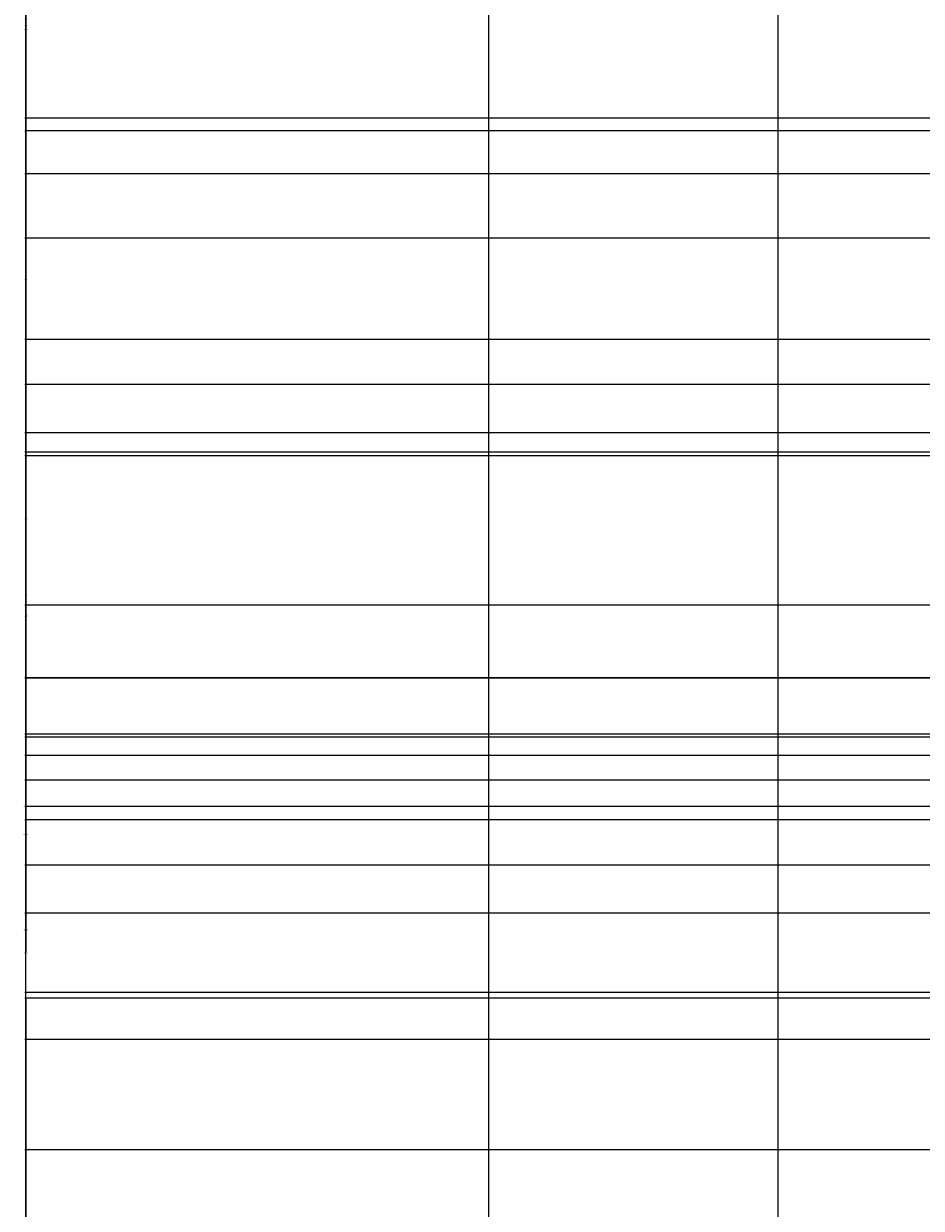
# Model space of a CAD drawing. Units: inches. Extents: x 818 to 1898, y 976 to 2364.
# Tile 5 of 96: x 818 to 986, y 1446 to 1668. Entities that reach past the tile are written whole.
import ezdxf

# ---------------------------------------------------------------- set-up
doc = ezdxf.new("R2010")
doc.units = ezdxf.units.IN
doc.header["$LTSCALE"] = 5
doc.header["$MEASUREMENT"] = 0
doc.layers.add('A-ANNO-DIMS', color=2, linetype='Continuous', lineweight=18)
doc.styles.get("Standard").update_dxf_attribs({"font": 'arial.ttf'})
doc.dimstyles.get("Standard").update_dxf_attribs({"dimtxt": 0.18, "dimasz": 0.18, "dimexe": 0.18, "dimexo": 0.0625, "dimgap": 0.09, "dimtad": 0, "dimtih": 1, "dimtoh": 1, "dimdec": 4, "dimzin": 0, "dimdsep": 46, "dimtxsty": 'Standard', "dimcen": 0.09, "dimadec": 0, "dimazin": 0, "dimtfac": 1, "dimtdec": 4, "dimtofl": 0, "dimtmove": 0, "dimatfit": 3, "dimfxl": 1, "dimtolj": 1, "dimtzin": 0, "dimarcsym": 0})

# ---------------------------------------------------------------- blocks, each defined once
blk = doc.blocks.new('*D59')
at = {"layer": 'A-ANNO-DIMS', "color": 0, "lineweight": -2, "ltscale": 5, "transparency": 16777216}
for p, q in [((1251.64, 2300.39), (818.03, 2300.39)), ((818.21, 2300.21), (818.21, 1669.95)), ((818.21, 1039.32), (818.21, 1669.59)), ((896.05, 1039.14), (818.03, 1039.14))]:
    blk.add_line(p, q, dxfattribs=at)
at = {"layer": 'A-ANNO-DIMS', "color": 0, "ltscale": 5, "transparency": 16777216}
for points in [[(818.18, 2300.21), (818.24, 2300.21), (818.21, 2300.39)], [(818.18, 1039.32), (818.24, 1039.32), (818.21, 1039.14)]]:
    blk.add_solid(points, dxfattribs=at)
at = {"layer": 'Defpoints', "color": 0, "ltscale": 5, "transparency": 16777216}
for p in [(818.21, 2300.39), (1251.71, 2300.39), (896.11, 1039.14)]:
    blk.add_point(p, dxfattribs=at)
at = {"layer": 'A-ANNO-DIMS', "color": 0, "ltscale": 5, "transparency": 16777216, "insert": (818.21, 1669.77), "char_height": 0.18, "attachment_point": 5}
blk.add_mtext('\\A1;1261.2', dxfattribs=at)
blk = doc.blocks.new('*D60')
at = {"layer": 'A-ANNO-DIMS', "color": 0, "lineweight": -2, "ltscale": 5, "transparency": 16777216}
for p, q in [((992.66, 2294.22), (818.03, 2294.22)), ((818.21, 2294.04), (818.21, 1748.77)), ((818.21, 1203.14), (818.21, 1748.41)), ((992.66, 1202.96), (818.03, 1202.96))]:
    blk.add_line(p, q, dxfattribs=at)
at = {"layer": 'A-ANNO-DIMS', "color": 0, "ltscale": 5, "transparency": 16777216}
for points in [[(818.18, 2294.04), (818.24, 2294.04), (818.21, 2294.22)], [(818.18, 1203.14), (818.24, 1203.14), (818.21, 1202.96)]]:
    blk.add_solid(points, dxfattribs=at)
at = {"layer": 'Defpoints', "color": 0, "ltscale": 5, "transparency": 16777216}
for p in [(818.21, 2294.22), (992.73, 2294.22), (992.73, 1202.96)]:
    blk.add_point(p, dxfattribs=at)
at = {"layer": 'A-ANNO-DIMS', "color": 0, "ltscale": 5, "transparency": 16777216, "insert": (818.21, 1748.59), "char_height": 0.18, "attachment_point": 5}
blk.add_mtext('\\A1;1091.3', dxfattribs=at)
blk = doc.blocks.new('*D63')
at = {"layer": 'A-ANNO-DIMS', "color": 0, "lineweight": -2, "ltscale": 5, "transparency": 16777216}
for p, q in [((1116.13, 1485.2), (818.03, 1485.2)), ((818.21, 1485.02), (818.21, 1360.77)), ((818.21, 1236.14), (818.21, 1360.4)), ((1116.13, 1235.96), (818.03, 1235.96))]:
    blk.add_line(p, q, dxfattribs=at)
at = {"layer": 'A-ANNO-DIMS', "color": 0, "ltscale": 5, "transparency": 16777216}
for points in [[(818.18, 1485.02), (818.24, 1485.02), (818.21, 1485.2)], [(818.18, 1236.14), (818.24, 1236.14), (818.21, 1235.96)]]:
    blk.add_solid(points, dxfattribs=at)
at = {"layer": 'Defpoints', "color": 0, "ltscale": 5, "transparency": 16777216}
for p in [(818.21, 1485.2), (1116.19, 1485.2), (1116.19, 1235.96)]:
    blk.add_point(p, dxfattribs=at)
at = {"layer": 'A-ANNO-DIMS', "color": 0, "ltscale": 5, "transparency": 16777216, "insert": (818.21, 1360.58), "char_height": 0.18, "attachment_point": 5}
blk.add_mtext('\\A1;249.24', dxfattribs=at)
blk = doc.blocks.new('*D84')
at = {"layer": 'A-ANNO-DIMS', "color": 0, "lineweight": -2, "ltscale": 5, "transparency": 16777216}
for p, q in [((1197.66, 1700.08), (818.03, 1700.08)), ((818.21, 1699.9), (818.21, 1600.76)), ((818.21, 1501.26), (818.21, 1600.4)), ((1197.66, 1501.08), (818.03, 1501.08))]:
    blk.add_line(p, q, dxfattribs=at)
at = {"layer": 'A-ANNO-DIMS', "color": 0, "ltscale": 5, "transparency": 16777216}
for points in [[(818.18, 1699.9), (818.24, 1699.9), (818.21, 1700.08)], [(818.18, 1501.26), (818.24, 1501.26), (818.21, 1501.08)]]:
    blk.add_solid(points, dxfattribs=at)
at = {"layer": 'Defpoints', "color": 0, "ltscale": 5, "transparency": 16777216}
for p in [(818.21, 1700.08), (1197.73, 1700.08), (1197.73, 1501.08)]:
    blk.add_point(p, dxfattribs=at)
at = {"layer": 'A-ANNO-DIMS', "color": 0, "ltscale": 5, "transparency": 16777216, "insert": (818.21, 1600.58), "char_height": 0.18, "attachment_point": 5}
blk.add_mtext('\\A1;199', dxfattribs=at)
blk = doc.blocks.new('*D90')
at = {"layer": 'A-ANNO-DIMS', "color": 0, "lineweight": -2, "ltscale": 5, "transparency": 16777216}
for p, q in [((904.95, 1071.12), (904.95, 2363.87)), ((905.13, 2363.69), (931.67, 2363.69)), ((958.99, 2363.69), (932.45, 2363.69)), ((959.17, 1071.12), (959.17, 2363.87))]:
    blk.add_line(p, q, dxfattribs=at)
at = {"layer": 'A-ANNO-DIMS', "color": 0, "ltscale": 5, "transparency": 16777216}
for points in [[(905.13, 2363.72), (905.13, 2363.66), (904.95, 2363.69)], [(958.99, 2363.72), (958.99, 2363.66), (959.17, 2363.69)]]:
    blk.add_solid(points, dxfattribs=at)
at = {"layer": 'Defpoints', "color": 0, "ltscale": 5, "transparency": 16777216}
for p in [(959.17, 2363.69), (904.95, 1071.06), (959.17, 1071.06)]:
    blk.add_point(p, dxfattribs=at)
at = {"layer": 'A-ANNO-DIMS', "color": 0, "ltscale": 5, "transparency": 16777216, "insert": (932.06, 2363.69), "char_height": 0.18, "attachment_point": 5}
blk.add_mtext('\\A1;54.22', dxfattribs=at)
blk = doc.blocks.new('*D91')
at = {"layer": 'A-ANNO-DIMS', "color": 0, "lineweight": -2, "ltscale": 5, "transparency": 16777216}
for p, q in [((959.17, 1071.12), (959.17, 2363.87)), ((959.35, 2363.69), (985.8, 2363.69)), ((1013.04, 2363.69), (986.59, 2363.69)), ((1013.22, 1071.12), (1013.22, 2363.87))]:
    blk.add_line(p, q, dxfattribs=at)
at = {"layer": 'A-ANNO-DIMS', "color": 0, "ltscale": 5, "transparency": 16777216}
for points in [[(959.35, 2363.72), (959.35, 2363.66), (959.17, 2363.69)], [(1013.04, 2363.72), (1013.04, 2363.66), (1013.22, 2363.69)]]:
    blk.add_solid(points, dxfattribs=at)
at = {"layer": 'Defpoints', "color": 0, "ltscale": 5, "transparency": 16777216}
for p in [(1013.22, 2363.69), (959.17, 1071.06), (1013.22, 1071.06)]:
    blk.add_point(p, dxfattribs=at)
at = {"layer": 'A-ANNO-DIMS', "color": 0, "ltscale": 5, "transparency": 16777216, "insert": (986.2, 2363.69), "char_height": 0.18, "attachment_point": 5}
blk.add_mtext('\\A1;54.04', dxfattribs=at)
blk = doc.blocks.new('*D116')
at = {"layer": 'A-ANNO-DIMS', "color": 0, "lineweight": -2, "ltscale": 5, "transparency": 16777216}
for p, q in [((1766.29, 1456.81), (818.03, 1456.81)), ((818.21, 1456.63), (818.21, 1417.41)), ((818.21, 1377.84), (818.21, 1417.05)), ((1766.29, 1377.66), (818.03, 1377.66))]:
    blk.add_line(p, q, dxfattribs=at)
at = {"layer": 'A-ANNO-DIMS', "color": 0, "ltscale": 5, "transparency": 16777216}
for points in [[(818.18, 1456.63), (818.24, 1456.63), (818.21, 1456.81)], [(818.18, 1377.84), (818.24, 1377.84), (818.21, 1377.66)]]:
    blk.add_solid(points, dxfattribs=at)
at = {"layer": 'Defpoints', "color": 0, "ltscale": 5, "transparency": 16777216}
for p in [(818.21, 1456.81), (1766.35, 1456.81), (1766.35, 1377.66)]:
    blk.add_point(p, dxfattribs=at)
at = {"layer": 'A-ANNO-DIMS', "color": 0, "ltscale": 5, "transparency": 16777216, "insert": (818.21, 1417.23), "char_height": 0.18, "attachment_point": 5}
blk.add_mtext('\\A1;79.15', dxfattribs=at)
blk = doc.blocks.new('*D117')
at = {"layer": 'A-ANNO-DIMS', "color": 0, "lineweight": -2, "ltscale": 5, "transparency": 16777216}
for p, q in [((1766.29, 1545.18), (818.03, 1545.18)), ((818.21, 1545), (818.21, 1501.18)), ((818.21, 1456.99), (818.21, 1500.81)), ((1766.29, 1456.81), (818.03, 1456.81))]:
    blk.add_line(p, q, dxfattribs=at)
at = {"layer": 'A-ANNO-DIMS', "color": 0, "ltscale": 5, "transparency": 16777216}
for points in [[(818.18, 1545), (818.24, 1545), (818.21, 1545.18)], [(818.18, 1456.99), (818.24, 1456.99), (818.21, 1456.81)]]:
    blk.add_solid(points, dxfattribs=at)
at = {"layer": 'Defpoints', "color": 0, "ltscale": 5, "transparency": 16777216}
for p in [(818.21, 1545.18), (1766.35, 1545.18), (1766.35, 1456.81)]:
    blk.add_point(p, dxfattribs=at)
at = {"layer": 'A-ANNO-DIMS', "color": 0, "ltscale": 5, "transparency": 16777216, "insert": (818.21, 1501), "char_height": 0.18, "attachment_point": 5}
blk.add_mtext('\\A1;88.37', dxfattribs=at)
blk = doc.blocks.new('*D118')
at = {"layer": 'A-ANNO-DIMS', "color": 0, "lineweight": -2, "ltscale": 5, "transparency": 16777216}
for p, q in [((1766.29, 1627.51), (818.03, 1627.51)), ((818.21, 1627.33), (818.21, 1586.53)), ((818.21, 1545.36), (818.21, 1586.16)), ((1766.29, 1545.18), (818.03, 1545.18))]:
    blk.add_line(p, q, dxfattribs=at)
at = {"layer": 'A-ANNO-DIMS', "color": 0, "ltscale": 5, "transparency": 16777216}
for points in [[(818.18, 1627.33), (818.24, 1627.33), (818.21, 1627.51)], [(818.18, 1545.36), (818.24, 1545.36), (818.21, 1545.18)]]:
    blk.add_solid(points, dxfattribs=at)
at = {"layer": 'Defpoints', "color": 0, "ltscale": 5, "transparency": 16777216}
for p in [(818.21, 1627.51), (1766.35, 1627.51), (1766.35, 1545.18)]:
    blk.add_point(p, dxfattribs=at)
at = {"layer": 'A-ANNO-DIMS', "color": 0, "ltscale": 5, "transparency": 16777216, "insert": (818.21, 1586.34), "char_height": 0.18, "attachment_point": 5}
blk.add_mtext('\\A1;82.32', dxfattribs=at)
blk = doc.blocks.new('*D119')
at = {"layer": 'A-ANNO-DIMS', "color": 0, "lineweight": -2, "ltscale": 5, "transparency": 16777216}
for p, q in [((1766.29, 1716.99), (818.03, 1716.99)), ((818.21, 1716.81), (818.21, 1672.43)), ((818.21, 1627.69), (818.21, 1672.06)), ((1766.29, 1627.51), (818.03, 1627.51))]:
    blk.add_line(p, q, dxfattribs=at)
at = {"layer": 'A-ANNO-DIMS', "color": 0, "ltscale": 5, "transparency": 16777216}
for points in [[(818.18, 1716.81), (818.24, 1716.81), (818.21, 1716.99)], [(818.18, 1627.69), (818.24, 1627.69), (818.21, 1627.51)]]:
    blk.add_solid(points, dxfattribs=at)
at = {"layer": 'Defpoints', "color": 0, "ltscale": 5, "transparency": 16777216}
for p in [(818.21, 1716.99), (1766.35, 1716.99), (1766.35, 1627.51)]:
    blk.add_point(p, dxfattribs=at)
at = {"layer": 'A-ANNO-DIMS', "color": 0, "ltscale": 5, "transparency": 16777216, "insert": (818.21, 1672.25), "char_height": 0.18, "attachment_point": 5}
blk.add_mtext('\\A1;89.48', dxfattribs=at)
blk = doc.blocks.new('*D129')
at = {"layer": 'A-ANNO-DIMS', "color": 0, "lineweight": -2, "ltscale": 5, "transparency": 16777216}
for p, q in [((1044.78, 1608.51), (818.03, 1608.51)), ((818.21, 1608.33), (818.21, 1521.27)), ((818.21, 1433.85), (818.21, 1520.91)), ((1044.78, 1433.67), (818.03, 1433.67))]:
    blk.add_line(p, q, dxfattribs=at)
at = {"layer": 'A-ANNO-DIMS', "color": 0, "ltscale": 5, "transparency": 16777216}
for points in [[(818.18, 1608.33), (818.24, 1608.33), (818.21, 1608.51)], [(818.18, 1433.85), (818.24, 1433.85), (818.21, 1433.67)]]:
    blk.add_solid(points, dxfattribs=at)
at = {"layer": 'Defpoints', "color": 0, "ltscale": 5, "transparency": 16777216}
for p in [(818.21, 1608.51), (1044.85, 1608.51), (1044.85, 1433.67)]:
    blk.add_point(p, dxfattribs=at)
at = {"layer": 'A-ANNO-DIMS', "color": 0, "ltscale": 5, "transparency": 16777216, "insert": (818.21, 1521.09), "char_height": 0.18, "attachment_point": 5}
blk.add_mtext('\\A1;174.84', dxfattribs=at)
blk = doc.blocks.new('*D130')
at = {"layer": 'A-ANNO-DIMS', "color": 0, "lineweight": -2, "ltscale": 5, "transparency": 16777216}
for p, q in [((1044.78, 1724.63), (818.03, 1724.63)), ((818.21, 1724.45), (818.21, 1666.75)), ((818.21, 1608.69), (818.21, 1666.39)), ((1044.78, 1608.51), (818.03, 1608.51))]:
    blk.add_line(p, q, dxfattribs=at)
at = {"layer": 'A-ANNO-DIMS', "color": 0, "ltscale": 5, "transparency": 16777216}
for points in [[(818.18, 1724.45), (818.24, 1724.45), (818.21, 1724.63)], [(818.18, 1608.69), (818.24, 1608.69), (818.21, 1608.51)]]:
    blk.add_solid(points, dxfattribs=at)
at = {"layer": 'Defpoints', "color": 0, "ltscale": 5, "transparency": 16777216}
for p in [(818.21, 1724.63), (1044.85, 1724.63), (1044.85, 1608.51)]:
    blk.add_point(p, dxfattribs=at)
at = {"layer": 'A-ANNO-DIMS', "color": 0, "ltscale": 5, "transparency": 16777216, "insert": (818.21, 1666.57), "char_height": 0.18, "attachment_point": 5}
blk.add_mtext('\\A1;116.12', dxfattribs=at)
blk = doc.blocks.new('*D156')
at = {"layer": 'A-ANNO-DIMS', "color": 0, "lineweight": -2, "ltscale": 5, "transparency": 16777216}
for p, q in [((1177.66, 1586.76), (818.03, 1586.76)), ((818.21, 1586.58), (818.21, 1560.86)), ((818.21, 1534.78), (818.21, 1560.5)), ((1177.66, 1534.6), (818.03, 1534.6))]:
    blk.add_line(p, q, dxfattribs=at)
at = {"layer": 'A-ANNO-DIMS', "color": 0, "ltscale": 5, "transparency": 16777216}
for points in [[(818.18, 1586.58), (818.24, 1586.58), (818.21, 1586.76)], [(818.18, 1534.78), (818.24, 1534.78), (818.21, 1534.6)]]:
    blk.add_solid(points, dxfattribs=at)
at = {"layer": 'Defpoints', "color": 0, "ltscale": 5, "transparency": 16777216}
for p in [(818.21, 1586.76), (1177.73, 1586.76), (1177.73, 1534.6)]:
    blk.add_point(p, dxfattribs=at)
at = {"layer": 'A-ANNO-DIMS', "color": 0, "ltscale": 5, "transparency": 16777216, "insert": (818.21, 1560.68), "char_height": 0.18, "attachment_point": 5}
blk.add_mtext('\\A1;52.16', dxfattribs=at)
blk = doc.blocks.new('*D157')
at = {"layer": 'A-ANNO-DIMS', "color": 0, "lineweight": -2, "ltscale": 5, "transparency": 16777216}
for p, q in [((1197.66, 1530.6), (818.03, 1530.6)), ((818.21, 1530.42), (818.21, 1516.02)), ((818.21, 1501.26), (818.21, 1515.66)), ((1197.66, 1501.08), (818.03, 1501.08))]:
    blk.add_line(p, q, dxfattribs=at)
at = {"layer": 'A-ANNO-DIMS', "color": 0, "ltscale": 5, "transparency": 16777216}
for points in [[(818.18, 1530.42), (818.24, 1530.42), (818.21, 1530.6)], [(818.18, 1501.26), (818.24, 1501.26), (818.21, 1501.08)]]:
    blk.add_solid(points, dxfattribs=at)
at = {"layer": 'Defpoints', "color": 0, "ltscale": 5, "transparency": 16777216}
for p in [(818.21, 1530.6), (1197.73, 1530.6), (1197.73, 1501.08)]:
    blk.add_point(p, dxfattribs=at)
at = {"layer": 'A-ANNO-DIMS', "color": 0, "ltscale": 5, "transparency": 16777216, "insert": (818.21, 1515.84), "char_height": 0.18, "attachment_point": 5}
blk.add_mtext('\\A1;29.524', dxfattribs=at)
blk = doc.blocks.new('*D168')
at = {"layer": 'A-ANNO-DIMS', "color": 0, "lineweight": -2, "ltscale": 5, "transparency": 16777216}
for p, q in [((1430.66, 1501.08), (818.03, 1501.08)), ((818.21, 1500.9), (818.21, 1493.84)), ((818.21, 1486.42), (818.21, 1493.48)), ((1430.66, 1486.24), (818.03, 1486.24))]:
    blk.add_line(p, q, dxfattribs=at)
at = {"layer": 'A-ANNO-DIMS', "color": 0, "ltscale": 5, "transparency": 16777216}
for points in [[(818.18, 1500.9), (818.24, 1500.9), (818.21, 1501.08)], [(818.18, 1486.42), (818.24, 1486.42), (818.21, 1486.24)]]:
    blk.add_solid(points, dxfattribs=at)
at = {"layer": 'Defpoints', "color": 0, "ltscale": 5, "transparency": 16777216}
for p in [(818.21, 1501.08), (1430.73, 1501.08), (1430.73, 1486.24)]:
    blk.add_point(p, dxfattribs=at)
at = {"layer": 'A-ANNO-DIMS', "color": 0, "ltscale": 5, "transparency": 16777216, "insert": (818.21, 1493.66), "char_height": 0.18, "attachment_point": 5}
blk.add_mtext('\\A1;14.84', dxfattribs=at)
blk = doc.blocks.new('*D176')
at = {"layer": 'A-ANNO-DIMS', "color": 0, "lineweight": -2, "ltscale": 5, "transparency": 16777216}
for p, q in [((1559.66, 1687.08), (818.03, 1687.08)), ((818.21, 1686.9), (818.21, 1667.51)), ((818.21, 1647.76), (818.21, 1667.15)), ((1559.66, 1647.58), (818.03, 1647.58))]:
    blk.add_line(p, q, dxfattribs=at)
at = {"layer": 'A-ANNO-DIMS', "color": 0, "ltscale": 5, "transparency": 16777216}
for points in [[(818.18, 1686.9), (818.24, 1686.9), (818.21, 1687.08)], [(818.18, 1647.76), (818.24, 1647.76), (818.21, 1647.58)]]:
    blk.add_solid(points, dxfattribs=at)
at = {"layer": 'Defpoints', "color": 0, "ltscale": 5, "transparency": 16777216}
for p in [(1559.73, 1687.08), (818.21, 1647.58), (1559.73, 1647.58)]:
    blk.add_point(p, dxfattribs=at)
at = {"layer": 'A-ANNO-DIMS', "color": 0, "ltscale": 5, "transparency": 16777216, "insert": (818.21, 1667.33), "char_height": 0.18, "attachment_point": 5}
blk.add_mtext('\\A1;39.5', dxfattribs=at)
blk = doc.blocks.new('*D181')
at = {"layer": 'A-ANNO-DIMS', "color": 0, "lineweight": -2, "ltscale": 5, "transparency": 16777216}
for p, q in [((1599.66, 1639.58), (818.03, 1639.58)), ((818.21, 1639.4), (818.21, 1620.01)), ((818.21, 1600.26), (818.21, 1619.65)), ((1619.66, 1600.08), (818.03, 1600.08))]:
    blk.add_line(p, q, dxfattribs=at)
at = {"layer": 'A-ANNO-DIMS', "color": 0, "ltscale": 5, "transparency": 16777216}
for points in [[(818.18, 1639.4), (818.24, 1639.4), (818.21, 1639.58)], [(818.18, 1600.26), (818.24, 1600.26), (818.21, 1600.08)]]:
    blk.add_solid(points, dxfattribs=at)
at = {"layer": 'Defpoints', "color": 0, "ltscale": 5, "transparency": 16777216}
for p in [(1599.73, 1639.58), (818.21, 1600.08), (1619.73, 1600.08)]:
    blk.add_point(p, dxfattribs=at)
at = {"layer": 'A-ANNO-DIMS', "color": 0, "ltscale": 5, "transparency": 16777216, "insert": (818.21, 1619.83), "char_height": 0.18, "attachment_point": 5}
blk.add_mtext('\\A1;39.5', dxfattribs=at)
blk = doc.blocks.new('*D187')
at = {"layer": 'A-ANNO-DIMS', "color": 0, "lineweight": -2, "ltscale": 5, "transparency": 16777216}
for p, q in [((1705.66, 1545.08), (818.03, 1545.08)), ((818.21, 1544.9), (818.21, 1533.26)), ((818.21, 1521.26), (818.21, 1532.9)), ((1705.66, 1521.08), (818.03, 1521.08))]:
    blk.add_line(p, q, dxfattribs=at)
at = {"layer": 'A-ANNO-DIMS', "color": 0, "ltscale": 5, "transparency": 16777216}
for points in [[(818.18, 1544.9), (818.24, 1544.9), (818.21, 1545.08)], [(818.18, 1521.26), (818.24, 1521.26), (818.21, 1521.08)]]:
    blk.add_solid(points, dxfattribs=at)
at = {"layer": 'Defpoints', "color": 0, "ltscale": 5, "transparency": 16777216}
for p in [(818.21, 1545.08), (1705.73, 1545.08), (1705.73, 1521.08)]:
    blk.add_point(p, dxfattribs=at)
at = {"layer": 'A-ANNO-DIMS', "color": 0, "ltscale": 5, "transparency": 16777216, "insert": (818.21, 1533.08), "char_height": 0.18, "attachment_point": 5}
blk.add_mtext('\\A1;24', dxfattribs=at)
blk = doc.blocks.new('*D194')
at = {"layer": 'A-ANNO-DIMS', "color": 0, "lineweight": -2, "ltscale": 5, "transparency": 16777216}
for p, q in [((1616.66, 1591.08), (818.03, 1591.08)), ((818.21, 1590.9), (818.21, 1575.1)), ((818.21, 1558.93), (818.21, 1574.73)), ((1616.66, 1558.75), (818.03, 1558.75))]:
    blk.add_line(p, q, dxfattribs=at)
at = {"layer": 'A-ANNO-DIMS', "color": 0, "ltscale": 5, "transparency": 16777216}
for points in [[(818.18, 1590.9), (818.24, 1590.9), (818.21, 1591.08)], [(818.18, 1558.93), (818.24, 1558.93), (818.21, 1558.75)]]:
    blk.add_solid(points, dxfattribs=at)
at = {"layer": 'Defpoints', "color": 0, "ltscale": 5, "transparency": 16777216}
for p in [(818.21, 1591.08), (1616.73, 1591.08), (1616.73, 1558.75)]:
    blk.add_point(p, dxfattribs=at)
at = {"layer": 'A-ANNO-DIMS', "color": 0, "ltscale": 5, "transparency": 16777216, "insert": (818.21, 1574.92), "char_height": 0.18, "attachment_point": 5}
blk.add_mtext('\\A1;32.326', dxfattribs=at)
blk = doc.blocks.new('*D201')
at = {"layer": 'A-ANNO-DIMS', "color": 0, "lineweight": -2, "ltscale": 5, "transparency": 16777216}
for p, q in [((1678.27, 1518.56), (818.03, 1518.56)), ((818.21, 1518.38), (818.21, 1498.18)), ((818.21, 1477.61), (818.21, 1497.81)), ((1678.27, 1477.43), (818.03, 1477.43))]:
    blk.add_line(p, q, dxfattribs=at)
at = {"layer": 'A-ANNO-DIMS', "color": 0, "ltscale": 5, "transparency": 16777216}
for points in [[(818.18, 1518.38), (818.24, 1518.38), (818.21, 1518.56)], [(818.18, 1477.61), (818.24, 1477.61), (818.21, 1477.43)]]:
    blk.add_solid(points, dxfattribs=at)
at = {"layer": 'Defpoints', "color": 0, "ltscale": 5, "transparency": 16777216}
for p in [(818.21, 1518.56), (1678.33, 1518.56), (1678.33, 1477.43)]:
    blk.add_point(p, dxfattribs=at)
at = {"layer": 'A-ANNO-DIMS', "color": 0, "ltscale": 5, "transparency": 16777216, "insert": (818.21, 1497.99), "char_height": 0.18, "attachment_point": 5}
blk.add_mtext('\\A1;41.135', dxfattribs=at)
blk = doc.blocks.new('*D270')
at = {"layer": 'A-ANNO-DIMS', "color": 0, "lineweight": -2, "ltscale": 5, "transparency": 16777216}
for p, q in [((1246.88, 1534.08), (818.03, 1534.08)), ((818.21, 1533.9), (818.21, 1522.26)), ((818.21, 1510.26), (818.21, 1521.9)), ((1246.88, 1510.08), (818.03, 1510.08))]:
    blk.add_line(p, q, dxfattribs=at)
at = {"layer": 'A-ANNO-DIMS', "color": 0, "ltscale": 5, "transparency": 16777216}
for points in [[(818.18, 1533.9), (818.24, 1533.9), (818.21, 1534.08)], [(818.18, 1510.26), (818.24, 1510.26), (818.21, 1510.08)]]:
    blk.add_solid(points, dxfattribs=at)
at = {"layer": 'Defpoints', "color": 0, "ltscale": 5, "transparency": 16777216}
for p in [(818.21, 1534.08), (1246.94, 1534.08), (1246.94, 1510.08)]:
    blk.add_point(p, dxfattribs=at)
at = {"layer": 'A-ANNO-DIMS', "color": 0, "ltscale": 5, "transparency": 16777216, "insert": (818.21, 1522.08), "char_height": 0.18, "attachment_point": 5}
blk.add_mtext('\\A1;24', dxfattribs=at)
blk = doc.blocks.new('*D272')
at = {"layer": 'A-ANNO-DIMS', "color": 0, "lineweight": -2, "ltscale": 5, "transparency": 16777216}
for p, q in [((1406.66, 1587.42), (818.03, 1587.42)), ((818.21, 1587.24), (818.21, 1556.89)), ((818.21, 1526.18), (818.21, 1556.52)), ((1406.66, 1526), (818.03, 1526))]:
    blk.add_line(p, q, dxfattribs=at)
at = {"layer": 'A-ANNO-DIMS', "color": 0, "ltscale": 5, "transparency": 16777216}
for points in [[(818.18, 1587.24), (818.24, 1587.24), (818.21, 1587.42)], [(818.18, 1526.18), (818.24, 1526.18), (818.21, 1526)]]:
    blk.add_solid(points, dxfattribs=at)
at = {"layer": 'Defpoints', "color": 0, "ltscale": 5, "transparency": 16777216}
for p in [(818.21, 1587.42), (1406.73, 1587.42), (1406.73, 1526)]:
    blk.add_point(p, dxfattribs=at)
at = {"layer": 'A-ANNO-DIMS', "color": 0, "ltscale": 5, "transparency": 16777216, "insert": (818.21, 1556.71), "char_height": 0.18, "attachment_point": 5}
blk.add_mtext('\\A1;61.42', dxfattribs=at)
blk = doc.blocks.new('*D277')
at = {"layer": 'A-ANNO-DIMS', "color": 0, "lineweight": -2, "ltscale": 5, "transparency": 16777216}
for p, q in [((1251.87, 1687.08), (818.03, 1687.08)), ((818.21, 1686.9), (818.21, 1668.7)), ((818.21, 1650.13), (818.21, 1668.33)), ((1256.59, 1649.95), (818.03, 1649.95))]:
    blk.add_line(p, q, dxfattribs=at)
at = {"layer": 'A-ANNO-DIMS', "color": 0, "ltscale": 5, "transparency": 16777216}
for points in [[(818.18, 1686.9), (818.24, 1686.9), (818.21, 1687.08)], [(818.18, 1650.13), (818.24, 1650.13), (818.21, 1649.95)]]:
    blk.add_solid(points, dxfattribs=at)
at = {"layer": 'Defpoints', "color": 0, "ltscale": 5, "transparency": 16777216}
for p in [(818.21, 1687.08), (1251.93, 1687.08), (1256.65, 1649.95)]:
    blk.add_point(p, dxfattribs=at)
at = {"layer": 'A-ANNO-DIMS', "color": 0, "ltscale": 5, "transparency": 16777216, "insert": (818.21, 1668.52), "char_height": 0.18, "attachment_point": 5}
blk.add_mtext('\\A1;37.13', dxfattribs=at)

msp = doc.modelspace()

# ---------------------------------------------------------------- dimensions: what is measured, and where the dimension line sits
at = {"layer": 'A-ANNO-DIMS', "ltscale": 5}
for base, p1, p2, picture, middle in [((959.1737, 2363.6929), (904.9504, 1071.0552), (959.1737, 1071.0552), '*D90', (932.062, 2363.6929)), ((1013.2176, 2363.6929), (959.1737, 1071.0552), (1013.2176, 1071.0552), '*D91', (986.1956, 2363.6929))]:
    dim = msp.add_linear_dim(base=base, p1=p1, p2=p2, dimstyle='Standard', override={"dimdec": 2, "dimlfac": 1, "dimrnd": 0, "dimzin": 0, "dimdsep": 46, "dimlunit": 2}, dxfattribs=at)
    dim.commit()
    dim.dimension.update_dxf_attribs({"geometry": picture, "text_midpoint": middle})
for base, p1, p2, override, picture, middle in [((818.2059, 2300.3929), (896.1138, 1039.1433), (1251.7057, 2300.3929), {"dimdec": 1, "dimlfac": 1, "dimrnd": 0, "dimzin": 0, "dimdsep": 46, "dimlunit": 2}, '*D59', (818.2059, 1669.7681)), ((818.2059, 2294.2171), (992.7251, 1202.9642), (992.7251, 2294.2171), {"dimdec": 1, "dimlfac": 1, "dimrnd": 0, "dimzin": 0, "dimdsep": 46, "dimlunit": 2}, '*D60', (818.2059, 1748.5907)), ((818.2059, 1724.63), (1044.8463, 1608.5116), (1044.8463, 1724.63), {"dimdec": 2, "dimlfac": 1, "dimrnd": 0, "dimzin": 0, "dimdsep": 46, "dimlunit": 2}, '*D130', (818.2059, 1666.5708)), ((818.2059, 1716.9866), (1766.3524, 1627.5052), (1766.3524, 1716.9866), {"dimdec": 2, "dimlfac": 1, "dimrnd": 0, "dimzin": 0, "dimdsep": 46, "dimlunit": 2}, '*D119', (818.2059, 1672.2459)), ((818.2059, 1700.0782), (1197.7251, 1501.0782), (1197.7251, 1700.0782), {"dimdec": 0, "dimlfac": 1, "dimrnd": 0, "dimzin": 0, "dimdsep": 46, "dimlunit": 2}, '*D84', (818.2059, 1600.5782)), ((818.2059, 1687.0782), (1256.6519, 1649.9518), (1251.9333, 1687.0782), {"dimdec": 2, "dimlfac": 1, "dimrnd": 0, "dimzin": 0, "dimdsep": 46, "dimlunit": 2}, '*D277', (818.2059, 1668.515)), ((818.2059, 1647.5782), (1559.7251, 1687.0782), (1559.7251, 1647.5782), {"dimdec": 1, "dimlfac": 1, "dimrnd": 0, "dimzin": 0, "dimdsep": 46, "dimlunit": 2}, '*D176', (818.2059, 1667.3282)), ((818.2059, 1600.0782), (1599.7251, 1639.5782), (1619.7251, 1600.0782), {"dimdec": 1, "dimlfac": 1, "dimrnd": 0, "dimzin": 0, "dimdsep": 46, "dimlunit": 2}, '*D181', (818.2059, 1619.8282)), ((818.2059, 1627.5052), (1766.3524, 1545.1827), (1766.3524, 1627.5052), {"dimdec": 2, "dimlfac": 1, "dimrnd": 0, "dimzin": 0, "dimdsep": 46, "dimlunit": 2}, '*D118', (818.2059, 1586.3439)), ((818.2059, 1608.5116), (1044.8463, 1433.6672), (1044.8463, 1608.5116), {"dimdec": 2, "dimlfac": 1, "dimrnd": 0, "dimzin": 0, "dimdsep": 46, "dimlunit": 2}, '*D129', (818.2059, 1521.0894)), ((818.2059, 1591.0782), (1616.7251, 1558.7521), (1616.7251, 1591.0782), {"dimdec": 3, "dimlfac": 1, "dimrnd": 0, "dimzin": 0, "dimdsep": 46, "dimlunit": 2}, '*D194', (818.2059, 1574.9152)), ((818.2059, 1587.4164), (1406.7251, 1525.9965), (1406.7251, 1587.4164), {"dimdec": 2, "dimlfac": 1, "dimrnd": 0, "dimzin": 0, "dimdsep": 46, "dimlunit": 2}, '*D272', (818.2059, 1556.7064)), ((818.2059, 1586.7585), (1177.7251, 1534.6024), (1177.7251, 1586.7585), {"dimdec": 2, "dimlfac": 1, "dimrnd": 0, "dimzin": 0, "dimdsep": 46, "dimlunit": 2}, '*D156', (818.2059, 1560.6805)), ((818.2059, 1545.1827), (1766.3524, 1456.8088), (1766.3524, 1545.1827), {"dimdec": 2, "dimlfac": 1, "dimrnd": 0, "dimzin": 0, "dimdsep": 46, "dimlunit": 2}, '*D117', (818.2059, 1500.9957)), ((818.2059, 1545.0782), (1705.7251, 1521.0782), (1705.7251, 1545.0782), {"dimdec": 0, "dimlfac": 1, "dimrnd": 0, "dimzin": 0, "dimdsep": 46, "dimlunit": 2}, '*D187', (818.2059, 1533.0782)), ((818.2059, 1534.0782), (1246.9377, 1510.0782), (1246.9377, 1534.0782), {"dimdec": 0, "dimlfac": 1, "dimrnd": 0, "dimzin": 0, "dimdsep": 46, "dimlunit": 2}, '*D270', (818.2059, 1522.0782)), ((818.2059, 1530.6024), (1197.7251, 1501.0782), (1197.7251, 1530.6024), {"dimdec": 3, "dimlfac": 1, "dimrnd": 0, "dimzin": 0, "dimdsep": 46, "dimlunit": 2}, '*D157', (818.2059, 1515.8403)), ((818.2059, 1518.5611), (1678.3302, 1477.4261), (1678.3302, 1518.5611), {"dimdec": 3, "dimlfac": 1, "dimrnd": 0, "dimzin": 0, "dimdsep": 46, "dimlunit": 2}, '*D201', (818.2059, 1497.9936)), ((818.2059, 1501.0782), (1430.7251, 1486.2383), (1430.7251, 1501.0782), {"dimdec": 2, "dimlfac": 1, "dimrnd": 0, "dimzin": 0, "dimdsep": 46, "dimlunit": 2}, '*D168', (818.2059, 1493.6583)), ((818.2059, 1485.2035), (1116.1882, 1235.9642), (1116.1882, 1485.2035), {"dimdec": 2, "dimlfac": 1, "dimrnd": 0, "dimzin": 0, "dimdsep": 46, "dimlunit": 2}, '*D63', (818.2059, 1360.5839)), ((818.2059, 1456.8088), (1766.3524, 1377.6564), (1766.3524, 1456.8088), {"dimdec": 2, "dimlfac": 1, "dimrnd": 0, "dimzin": 0, "dimdsep": 46, "dimlunit": 2}, '*D116', (818.2059, 1417.2326))]:
    dim = msp.add_linear_dim(base=base, p1=p1, p2=p2, angle=90, dimstyle='Standard', override=override, dxfattribs=at)
    dim.commit()
    dim.dimension.update_dxf_attribs({"geometry": picture, "text_midpoint": middle})

doc.saveas('drawing.dxf')
